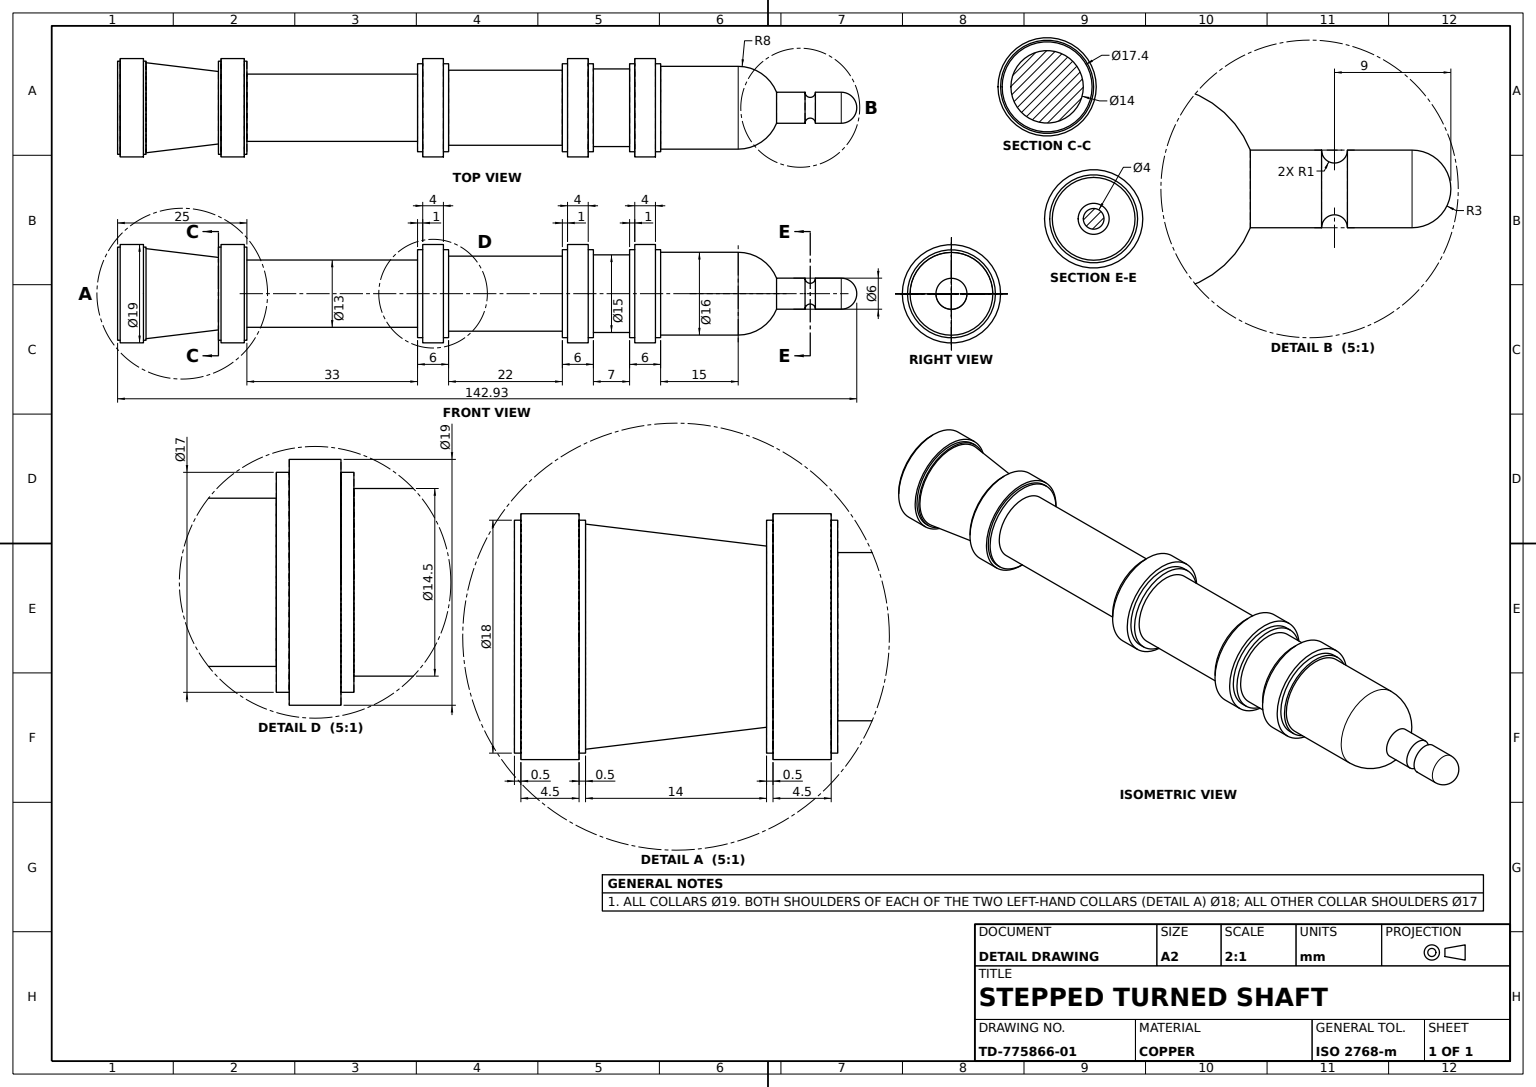
from build123d import *

# Parameters (mm, degrees)
MID_SECTION_PROFILE_W = 33
MID_SECTION_PROFILE_H = 6.5
TIP_DOME_FILLET_R8_R  = 8
END_FLARE_FILLET_R3_R = 3


with BuildPart() as part:
    # Shaft Core Profile → Shaft Core Revolve (revolve)
    with BuildSketch(Plane.XY, mode=Mode.PRIVATE) as shaft_core_revolve_sk:
        Polygon((0, 0), (0, 9), (0.5, 9), (0.5, 9.5), (5, 9.5), (5, 9), (5.5, 9), (5.5, 8.7), (19.5, 7), (19.5, 9), (20, 9), (20, 9.5), (24.5, 9.5), (24.5, 9), (25, 9), (25, 0), align=None)
    revolve(shaft_core_revolve_sk.sketch.rotate(Axis((0, 0, 0), (1, 0, 0)), 90), axis=Axis((0, 0, 0), (1, 0, 0)))

    # Mid Section Profile → Mid Section Revolve (revolve)
    with BuildSketch(Plane.XY, mode=Mode.PRIVATE) as mid_section_revolve_sk:
        with Locations((41.5, 3.25)):
            Rectangle(MID_SECTION_PROFILE_W, MID_SECTION_PROFILE_H)
    revolve(mid_section_revolve_sk.sketch.rotate(Axis((25, 0, 0), (1, 0, 0)), 90), axis=Axis((25, 0, 0), (1, 0, 0)))

    # Collars Profile → Collars Revolve (revolve)
    with BuildSketch(Plane.XY, mode=Mode.PRIVATE) as collars_revolve_sk:
        Polygon((58, 0), (58, 8.5), (59, 8.5), (59, 9.5), (63, 9.5), (63, 8.5), (64, 8.5), (64, 7.25), (86, 7.25), (86, 8.5), (87, 8.5), (87, 9.5), (91, 9.5), (91, 8.5), (92, 8.5), (92, 7.5), (99, 7.5), (99, 8.5), (100, 8.5), (100, 9.5), (104, 9.5), (104, 8.5), (105, 8.5), (105, 8), (120, 8), (128, 8), (128, 0), align=None)
    revolve(collars_revolve_sk.sketch.rotate(Axis((58, 0, 0), (1, 0, 0)), 90), axis=Axis((58, 0, 0), (1, 0, 0)))

    # Tip Dome Fillet R8
    tip_dome_fillet_r8_edges = [part.edges().sort_by_distance(p)[0] for p in [
        (128, 0, -8),
    ]]
    fillet(tip_dome_fillet_r8_edges, radius=TIP_DOME_FILLET_R8_R)

    # End Flare Profile → End Flare Revolve (revolve)
    with BuildSketch(Plane.XY, mode=Mode.PRIVATE) as end_flare_revolve_sk:
        with BuildLine():
            Line((124.926812112, 0), (124.926812112, 3))
            Line((124.926812112, 3), (132.926812112, 3))
            ThreePointArc((132.926812112, 3), (133.926812112, 2), (134.926812112, 3))
            Line((134.926812112, 3), (139.926812112, 3))
            Line((139.926812112, 3), (142.926812112, 3))
            Line((142.926812112, 3), (142.926812112, 0))
            Line((142.926812112, 0), (124.926812112, 0))
        make_face()
    revolve(end_flare_revolve_sk.sketch.rotate(Axis((124.926812112, 0, 0), (1, 0, 0)), 90), axis=Axis((124.926812112, 0, 0), (1, 0, 0)))

    # End Flare Fillet R3
    end_flare_fillet_r3_edges = [part.edges().sort_by_distance(p)[0] for p in [
        (142.926812112, 0, -3),
    ]]
    fillet(end_flare_fillet_r3_edges, radius=END_FLARE_FILLET_R3_R)


solid = part.part
